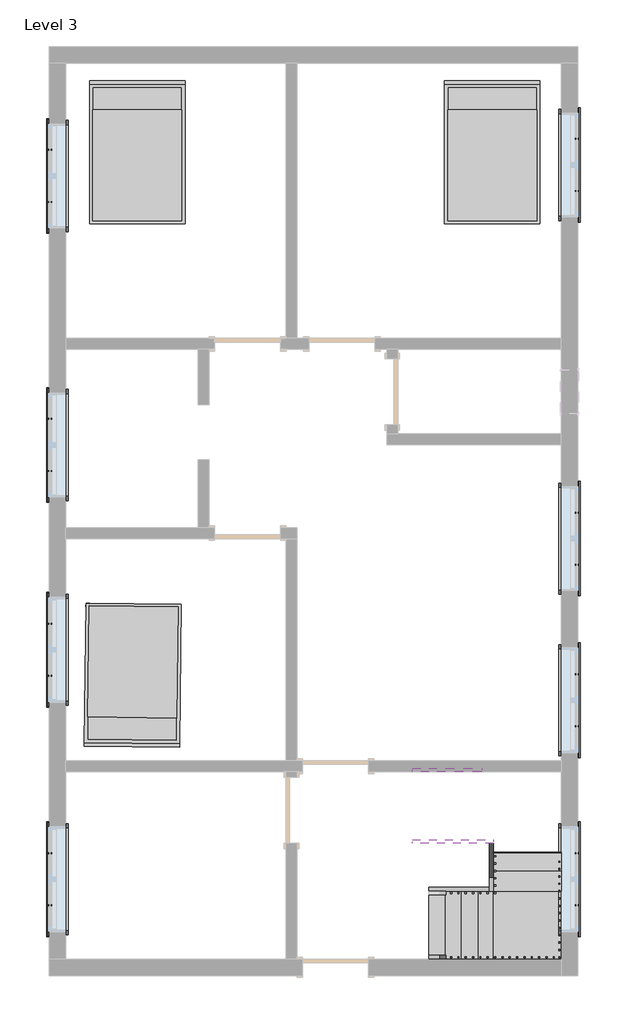
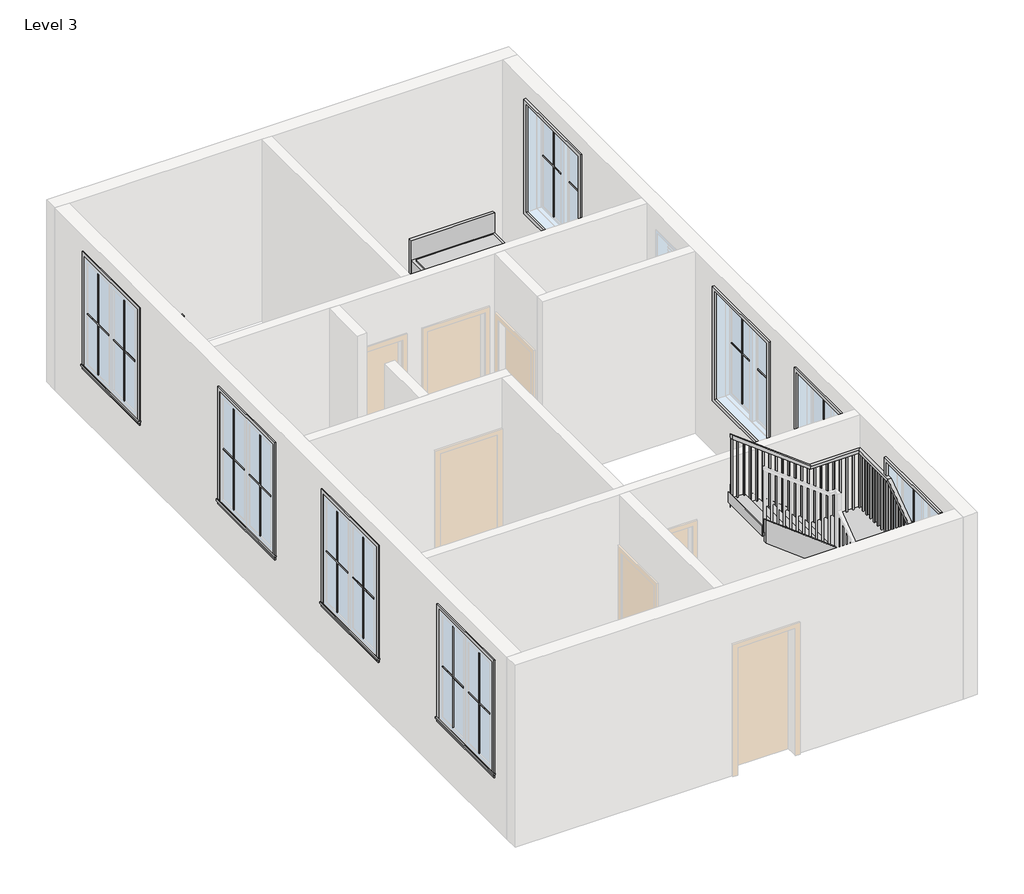
# One storey, part 2 of 2: 32 proxies, 5 members, 3 furniture elements, 1 railing, 1 stair flight.
"""IFC4 building model written with IfcOpenShell, lengths in millimetres."""

from ifc_helpers import new_model, si_unit, frame, origin, place, context, project, spatial, polyline, outline, extrude, faceted_brep, transform, mapped, element, save
from components import muntin_pattern_2x2_muntin_pattern_2x2_bff912c5, muntin_pattern_2x2_muntin_pattern_2x2_c2194282, trim_window_exterior_flat_with_sill_e04b3088, trim_window_interior_flat_picture_frame_2a7685fe, bed_17739_bed_17739_15c61121, stair_flight_84673ee4

model = new_model("IFC4")

# Units and contexts
model_context = context("Model", 3, world=origin())
ifc_project = project(units=[si_unit("LENGTHUNIT", "METRE", prefix="MILLI")], contexts=[model_context])

# Site, building, storey
site = spatial("IfcSite", under=ifc_project)
building = spatial("IfcBuilding", under=site)
storey = spatial("IfcBuildingStorey", under=building, Name="Level 3", Elevation=3200.4)

# Proxies
placement = place(None, origin())
muntin_pattern_2x2_muntin_pattern_2x2_shape = muntin_pattern_2x2_muntin_pattern_2x2_bff912c5(model_context)
element("IfcBuildingElementProxy", 1, Name="Muntin Pattern_2x2 : Muntin Pattern_2x2", ObjectType="Muntin Pattern_2x2 : Muntin Pattern_2x2", at=placement, inside=storey, context=model_context, shape_type="MappedRepresentation", body=[
    mapped(muntin_pattern_2x2_muntin_pattern_2x2_shape, transform((-4903.510885, -5396.5975571, 4184.65), x_axis=(0.0, 1.0, 0.0), y_axis=(-1.0, 0.0, 0.0), z_axis=(0.0, 0.0, 1.0))),
])
element("IfcBuildingElementProxy", 2, Name="Muntin Pattern_2x2 : Muntin Pattern_2x2", ObjectType="Muntin Pattern_2x2 : Muntin Pattern_2x2", at=placement, inside=storey, context=model_context, shape_type="MappedRepresentation", body=[
    mapped(muntin_pattern_2x2_muntin_pattern_2x2_shape, transform((2392.639115, -4675.8725571, 4184.65), x_axis=(0.0, -1.0, 0.0), y_axis=(1.0, 0.0, 0.0), z_axis=(0.0, 0.0, 1.0))),
])
element("IfcBuildingElementProxy", 3, Name="Muntin Pattern_2x2 : Muntin Pattern_2x2", ObjectType="Muntin Pattern_2x2 : Muntin Pattern_2x2", at=placement, inside=storey, context=model_context, shape_type="MappedRepresentation", body=[
    mapped(muntin_pattern_2x2_muntin_pattern_2x2_shape, transform((2392.639115, -2199.3725571, 4184.65), x_axis=(0.0, -1.0, 0.0), y_axis=(1.0, 0.0, 0.0), z_axis=(0.0, 0.0, 1.0))),
])
element("IfcBuildingElementProxy", 4, Name="Muntin Pattern_2x2 : Muntin Pattern_2x2", ObjectType="Muntin Pattern_2x2 : Muntin Pattern_2x2", at=placement, inside=storey, context=model_context, shape_type="MappedRepresentation", body=[
    mapped(muntin_pattern_2x2_muntin_pattern_2x2_shape, transform((2392.639115, 35.8274429, 4184.65), x_axis=(0.0, -1.0, 0.0), y_axis=(1.0, 0.0, 0.0), z_axis=(0.0, 0.0, 1.0))),
])
element("IfcBuildingElementProxy", 5, Name="Muntin Pattern_2x2 : Muntin Pattern_2x2", ObjectType="Muntin Pattern_2x2 : Muntin Pattern_2x2", at=placement, inside=storey, context=model_context, shape_type="MappedRepresentation", body=[
    mapped(muntin_pattern_2x2_muntin_pattern_2x2_shape, transform((-4903.510885, -2221.5975571, 4184.65), x_axis=(0.0, 1.0, 0.0), y_axis=(-1.0, 0.0, 0.0), z_axis=(0.0, 0.0, 1.0))),
])
element("IfcBuildingElementProxy", 6, Name="Muntin Pattern_2x2 : Muntin Pattern_2x2", ObjectType="Muntin Pattern_2x2 : Muntin Pattern_2x2", at=placement, inside=storey, context=model_context, shape_type="MappedRepresentation", body=[
    mapped(muntin_pattern_2x2_muntin_pattern_2x2_shape, transform((-4903.510885, 610.5024429, 4184.65), x_axis=(0.0, 1.0, 0.0), y_axis=(-1.0, 0.0, 0.0), z_axis=(0.0, 0.0, 1.0))),
])
element("IfcBuildingElementProxy", 7, Name="Muntin Pattern_2x2 : Muntin Pattern_2x2", ObjectType="Muntin Pattern_2x2 : Muntin Pattern_2x2", at=placement, inside=storey, context=model_context, shape_type="MappedRepresentation", body=[
    mapped(muntin_pattern_2x2_muntin_pattern_2x2_shape, transform((-4903.510885, 4331.6024429, 4184.65), x_axis=(0.0, 1.0, 0.0), y_axis=(-1.0, 0.0, 0.0), z_axis=(0.0, 0.0, 1.0))),
])
element("IfcBuildingElementProxy", 8, Name="Muntin Pattern_2x2 : Muntin Pattern_2x2", ObjectType="Muntin Pattern_2x2 : Muntin Pattern_2x2", at=placement, inside=storey, context=model_context, shape_type="MappedRepresentation", body=[
    mapped(muntin_pattern_2x2_muntin_pattern_2x2_shape, transform((2392.639115, 5204.7274429, 4184.65), x_axis=(0.0, -1.0, 0.0), y_axis=(1.0, 0.0, 0.0), z_axis=(0.0, 0.0, 1.0))),
])
muntin_pattern_2x2_muntin_pattern_2x2_2_shape = muntin_pattern_2x2_muntin_pattern_2x2_c2194282(model_context)
element("IfcBuildingElementProxy", 9, Name="Muntin Pattern_2x2 : Muntin Pattern_2x2", ObjectType="Muntin Pattern_2x2 : Muntin Pattern_2x2", at=placement, inside=storey, context=model_context, shape_type="MappedRepresentation", body=[
    mapped(muntin_pattern_2x2_muntin_pattern_2x2_2_shape, transform((-4903.510885, -4675.8725571, 4184.65), x_axis=(0.0, -1.0, 0.0), y_axis=(1.0, 0.0, 0.0), z_axis=(0.0, 0.0, 1.0))),
])
element("IfcBuildingElementProxy", 10, Name="Muntin Pattern_2x2 : Muntin Pattern_2x2", ObjectType="Muntin Pattern_2x2 : Muntin Pattern_2x2", at=placement, inside=storey, context=model_context, shape_type="MappedRepresentation", body=[
    mapped(muntin_pattern_2x2_muntin_pattern_2x2_2_shape, transform((2392.639115, -5396.5975571, 4184.65), x_axis=(0.0, 1.0, 0.0), y_axis=(-1.0, 0.0, 0.0), z_axis=(0.0, 0.0, 1.0))),
])
element("IfcBuildingElementProxy", 11, Name="Muntin Pattern_2x2 : Muntin Pattern_2x2", ObjectType="Muntin Pattern_2x2 : Muntin Pattern_2x2", at=placement, inside=storey, context=model_context, shape_type="MappedRepresentation", body=[
    mapped(muntin_pattern_2x2_muntin_pattern_2x2_2_shape, transform((2392.639115, -2920.0975571, 4184.65), x_axis=(0.0, 1.0, 0.0), y_axis=(-1.0, 0.0, 0.0), z_axis=(0.0, 0.0, 1.0))),
])
element("IfcBuildingElementProxy", 12, Name="Muntin Pattern_2x2 : Muntin Pattern_2x2", ObjectType="Muntin Pattern_2x2 : Muntin Pattern_2x2", at=placement, inside=storey, context=model_context, shape_type="MappedRepresentation", body=[
    mapped(muntin_pattern_2x2_muntin_pattern_2x2_2_shape, transform((2392.639115, -684.8975571, 4184.65), x_axis=(0.0, 1.0, 0.0), y_axis=(-1.0, 0.0, 0.0), z_axis=(0.0, 0.0, 1.0))),
])
element("IfcBuildingElementProxy", 13, Name="Muntin Pattern_2x2 : Muntin Pattern_2x2", ObjectType="Muntin Pattern_2x2 : Muntin Pattern_2x2", at=placement, inside=storey, context=model_context, shape_type="MappedRepresentation", body=[
    mapped(muntin_pattern_2x2_muntin_pattern_2x2_2_shape, transform((-4903.510885, -1500.8725571, 4184.65), x_axis=(0.0, -1.0, 0.0), y_axis=(1.0, 0.0, 0.0), z_axis=(0.0, 0.0, 1.0))),
])
element("IfcBuildingElementProxy", 14, Name="Muntin Pattern_2x2 : Muntin Pattern_2x2", ObjectType="Muntin Pattern_2x2 : Muntin Pattern_2x2", at=placement, inside=storey, context=model_context, shape_type="MappedRepresentation", body=[
    mapped(muntin_pattern_2x2_muntin_pattern_2x2_2_shape, transform((-4903.510885, 1331.2274429, 4184.65), x_axis=(0.0, -1.0, 0.0), y_axis=(1.0, 0.0, 0.0), z_axis=(0.0, 0.0, 1.0))),
])
element("IfcBuildingElementProxy", 15, Name="Muntin Pattern_2x2 : Muntin Pattern_2x2", ObjectType="Muntin Pattern_2x2 : Muntin Pattern_2x2", at=placement, inside=storey, context=model_context, shape_type="MappedRepresentation", body=[
    mapped(muntin_pattern_2x2_muntin_pattern_2x2_2_shape, transform((-4903.510885, 5052.3274429, 4184.65), x_axis=(0.0, -1.0, 0.0), y_axis=(1.0, 0.0, 0.0), z_axis=(0.0, 0.0, 1.0))),
])
element("IfcBuildingElementProxy", 16, Name="Muntin Pattern_2x2 : Muntin Pattern_2x2", ObjectType="Muntin Pattern_2x2 : Muntin Pattern_2x2", at=placement, inside=storey, context=model_context, shape_type="MappedRepresentation", body=[
    mapped(muntin_pattern_2x2_muntin_pattern_2x2_2_shape, transform((2392.639115, 4484.0024429, 4184.65), x_axis=(0.0, 1.0, 0.0), y_axis=(-1.0, 0.0, 0.0), z_axis=(0.0, 0.0, 1.0))),
])
trim_window_exterior_flat_with_sill_shape = trim_window_exterior_flat_with_sill_e04b3088(model_context)
element("IfcBuildingElementProxy", 17, Name="Trim-Window-Exterior-Flat : with Sill", ObjectType="Trim-Window-Exterior-Flat : with Sill", at=placement, inside=storey, context=model_context, shape_type="MappedRepresentation", body=[
    mapped(trim_window_exterior_flat_with_sill_shape, transform((-4913.035885, -5036.2350571, 5943.6), x_axis=(0.0, -1.0, 0.0), y_axis=(0.0, 0.0, 1.0), z_axis=(-1.0, 0.0, 0.0))),
])
element("IfcBuildingElementProxy", 18, Name="Trim-Window-Exterior-Flat : with Sill", ObjectType="Trim-Window-Exterior-Flat : with Sill", at=placement, inside=storey, context=model_context, shape_type="MappedRepresentation", body=[
    mapped(trim_window_exterior_flat_with_sill_shape, transform((2402.164115, -5036.2350571, 5943.6), x_axis=(0.0, 1.0, 0.0), y_axis=(0.0, 0.0, 1.0), z_axis=(1.0, 0.0, 0.0))),
])
element("IfcBuildingElementProxy", 19, Name="Trim-Window-Exterior-Flat : with Sill", ObjectType="Trim-Window-Exterior-Flat : with Sill", at=placement, inside=storey, context=model_context, shape_type="MappedRepresentation", body=[
    mapped(trim_window_exterior_flat_with_sill_shape, transform((2402.164115, -2559.7350571, 5943.6), x_axis=(0.0, 1.0, 0.0), y_axis=(0.0, 0.0, 1.0), z_axis=(1.0, 0.0, 0.0))),
])
element("IfcBuildingElementProxy", 20, Name="Trim-Window-Exterior-Flat : with Sill", ObjectType="Trim-Window-Exterior-Flat : with Sill", at=placement, inside=storey, context=model_context, shape_type="MappedRepresentation", body=[
    mapped(trim_window_exterior_flat_with_sill_shape, transform((2402.164115, -324.5350571, 5943.6), x_axis=(0.0, 1.0, 0.0), y_axis=(0.0, 0.0, 1.0), z_axis=(1.0, 0.0, 0.0))),
])
element("IfcBuildingElementProxy", 21, Name="Trim-Window-Exterior-Flat : with Sill", ObjectType="Trim-Window-Exterior-Flat : with Sill", at=placement, inside=storey, context=model_context, shape_type="MappedRepresentation", body=[
    mapped(trim_window_exterior_flat_with_sill_shape, transform((-4913.035885, -1861.2350571, 5943.6), x_axis=(0.0, -1.0, 0.0), y_axis=(0.0, 0.0, 1.0), z_axis=(-1.0, 0.0, 0.0))),
])
element("IfcBuildingElementProxy", 22, Name="Trim-Window-Exterior-Flat : with Sill", ObjectType="Trim-Window-Exterior-Flat : with Sill", at=placement, inside=storey, context=model_context, shape_type="MappedRepresentation", body=[
    mapped(trim_window_exterior_flat_with_sill_shape, transform((-4913.035885, 970.8649429, 5943.6), x_axis=(0.0, -1.0, 0.0), y_axis=(0.0, 0.0, 1.0), z_axis=(-1.0, 0.0, 0.0))),
])
element("IfcBuildingElementProxy", 23, Name="Trim-Window-Exterior-Flat : with Sill", ObjectType="Trim-Window-Exterior-Flat : with Sill", at=placement, inside=storey, context=model_context, shape_type="MappedRepresentation", body=[
    mapped(trim_window_exterior_flat_with_sill_shape, transform((-4913.035885, 4691.9649429, 5943.6), x_axis=(0.0, -1.0, 0.0), y_axis=(0.0, 0.0, 1.0), z_axis=(-1.0, 0.0, 0.0))),
])
element("IfcBuildingElementProxy", 24, Name="Trim-Window-Exterior-Flat : with Sill", ObjectType="Trim-Window-Exterior-Flat : with Sill", at=placement, inside=storey, context=model_context, shape_type="MappedRepresentation", body=[
    mapped(trim_window_exterior_flat_with_sill_shape, transform((2402.164115, 4844.3649429, 5943.6), x_axis=(0.0, 1.0, 0.0), y_axis=(0.0, 0.0, 1.0), z_axis=(1.0, 0.0, 0.0))),
])
trim_window_interior_flat_picture_frame_shape = trim_window_interior_flat_picture_frame_2a7685fe(model_context)
element("IfcBuildingElementProxy", 25, Name="Trim-Window-Interior-Flat : Picture Frame", ObjectType="Trim-Window-Interior-Flat : Picture Frame", at=placement, inside=storey, context=model_context, shape_type="MappedRepresentation", body=[
    mapped(trim_window_interior_flat_picture_frame_shape, transform((-4684.435885, -5036.2350571, 5943.6), x_axis=(0.0, 1.0, 0.0), y_axis=(0.0, 0.0, 1.0), z_axis=(1.0, 0.0, 0.0))),
])
element("IfcBuildingElementProxy", 26, Name="Trim-Window-Interior-Flat : Picture Frame", ObjectType="Trim-Window-Interior-Flat : Picture Frame", at=placement, inside=storey, context=model_context, shape_type="MappedRepresentation", body=[
    mapped(trim_window_interior_flat_picture_frame_shape, transform((2173.564115, -5036.2350571, 5943.6), x_axis=(0.0, -1.0, 0.0), y_axis=(0.0, 0.0, 1.0), z_axis=(-1.0, 0.0, 0.0))),
])
element("IfcBuildingElementProxy", 27, Name="Trim-Window-Interior-Flat : Picture Frame", ObjectType="Trim-Window-Interior-Flat : Picture Frame", at=placement, inside=storey, context=model_context, shape_type="MappedRepresentation", body=[
    mapped(trim_window_interior_flat_picture_frame_shape, transform((2173.564115, -2559.7350571, 5943.6), x_axis=(0.0, -1.0, 0.0), y_axis=(0.0, 0.0, 1.0), z_axis=(-1.0, 0.0, 0.0))),
])
element("IfcBuildingElementProxy", 28, Name="Trim-Window-Interior-Flat : Picture Frame", ObjectType="Trim-Window-Interior-Flat : Picture Frame", at=placement, inside=storey, context=model_context, shape_type="MappedRepresentation", body=[
    mapped(trim_window_interior_flat_picture_frame_shape, transform((2173.564115, -324.5350571, 5943.6), x_axis=(0.0, -1.0, 0.0), y_axis=(0.0, 0.0, 1.0), z_axis=(-1.0, 0.0, 0.0))),
])
element("IfcBuildingElementProxy", 29, Name="Trim-Window-Interior-Flat : Picture Frame", ObjectType="Trim-Window-Interior-Flat : Picture Frame", at=placement, inside=storey, context=model_context, shape_type="MappedRepresentation", body=[
    mapped(trim_window_interior_flat_picture_frame_shape, transform((-4684.435885, -1861.2350571, 5943.6), x_axis=(0.0, 1.0, 0.0), y_axis=(0.0, 0.0, 1.0), z_axis=(1.0, 0.0, 0.0))),
])
element("IfcBuildingElementProxy", 30, Name="Trim-Window-Interior-Flat : Picture Frame", ObjectType="Trim-Window-Interior-Flat : Picture Frame", at=placement, inside=storey, context=model_context, shape_type="MappedRepresentation", body=[
    mapped(trim_window_interior_flat_picture_frame_shape, transform((-4684.435885, 970.8649429, 5943.6), x_axis=(0.0, 1.0, 0.0), y_axis=(0.0, 0.0, 1.0), z_axis=(1.0, 0.0, 0.0))),
])
element("IfcBuildingElementProxy", 31, Name="Trim-Window-Interior-Flat : Picture Frame", ObjectType="Trim-Window-Interior-Flat : Picture Frame", at=placement, inside=storey, context=model_context, shape_type="MappedRepresentation", body=[
    mapped(trim_window_interior_flat_picture_frame_shape, transform((-4684.435885, 4691.9649429, 5943.6), x_axis=(0.0, 1.0, 0.0), y_axis=(0.0, 0.0, 1.0), z_axis=(1.0, 0.0, 0.0))),
])
element("IfcBuildingElementProxy", 32, Name="Trim-Window-Interior-Flat : Picture Frame", ObjectType="Trim-Window-Interior-Flat : Picture Frame", at=placement, inside=storey, context=model_context, shape_type="MappedRepresentation", body=[
    mapped(trim_window_interior_flat_picture_frame_shape, transform((2173.564115, 4844.3649429, 5943.6), x_axis=(0.0, -1.0, 0.0), y_axis=(0.0, 0.0, 1.0), z_axis=(-1.0, 0.0, 0.0))),
])

# Furniture
bed_17739_bed_17739_shape = bed_17739_bed_17739_15c61121(model_context)
element("IfcFurniture", 33, ObjectType="Bed_17739 : Bed_17739", at=placement, inside=storey, context=model_context, shape_type="MappedRepresentation", body=[
    mapped(bed_17739_bed_17739_shape, transform((-3693.835885, 4996.7649429, 3200.4), x_axis=(1.0, 0.0, 0.0), y_axis=(0.0, 1.0, 0.0), z_axis=(0.0, 0.0, 1.0))),
])
element("IfcFurniture", 34, ObjectType="Bed_17739 : Bed_17739", at=placement, inside=storey, context=model_context, shape_type="MappedRepresentation", body=[
    mapped(bed_17739_bed_17739_shape, transform((1221.064115, 4996.7649429, 3200.4), x_axis=(1.0, 0.0, 0.0), y_axis=(0.0, 1.0, 0.0), z_axis=(0.0, 0.0, 1.0))),
])
element("IfcFurniture", 35, ObjectType="Bed_17739 : Bed_17739", at=placement, inside=storey, context=model_context, shape_type="MappedRepresentation", body=[
    mapped(bed_17739_bed_17739_shape, transform((-3756.0321663, -2189.364606, 3200.4), x_axis=(-0.9999334593473937, 0.011535895177843815, 0.0), y_axis=(-0.011535895177843815, -0.9999334593473937, 0.0), z_axis=(0.0, 0.0, 1.0))),
])

# Members
element("IfcMember", 36, ObjectType="Stringer - 2\" Width", at=placement, inside=storey, context=model_context, shape_type="SweptSolid", body=[
    extrude(outline(polyline([(3423.0959685, 344.764115), (3200.4, 344.764115), (3200.4, 555.1685253), (3683.3196844, 1182.964115), (4067.8651993, 1182.964115), (3423.0959685, 344.764115)])), frame((0.0, -5201.3350571, 0.0), z_axis=(0.0, 1.0, 0.0), x_axis=(0.0, 0.0, 1.0)), (0.0, 0.0, 1.0), 50.8),
])
element("IfcMember", 37, ObjectType="Stringer - 2\" Width", at=placement, inside=storey, context=model_context, shape_type="SweptSolid", body=[
    extrude(outline(polyline([(-5201.3350571, 3895.552716), (-5201.3350571, 4270.1225362), (-4540.9350571, 4741.8368219), (-4540.9350571, 4367.2670017), (-5201.3350571, 3895.552716)])), frame((1182.964115, 0.0, 0.0), z_axis=(1.0, 0.0, 0.0), x_axis=(0.0, 1.0, 0.0)), (0.0, 0.0, 1.0), 50.8),
])
element("IfcMember", 38, ObjectType="Stringer - 2\" Width", at=placement, inside=storey, context=model_context, shape_type="SweptSolid", body=[
    extrude(outline(polyline([(4569.5786616, 1233.764115), (4952.7668, 1233.764115), (5804.2715619, 116.164115), (5421.0834236, 116.164115), (4569.5786616, 1233.764115)])), frame((0.0, -4540.9350571, 0.0), z_axis=(0.0, 1.0, 0.0), x_axis=(0.0, 0.0, 1.0)), (0.0, 0.0, 1.0), 50.8),
])
element("IfcMember", 39, ObjectType="Stringer - 2\" Width", at=placement, inside=storey, context=model_context, shape_type="SweptSolid", body=[
    extrude(outline(polyline([(3423.0959685, 344.764115), (3200.4, 344.764115), (3200.4, 555.1685253), (3598.8368219, 1073.1363938), (3598.8368219, 573.2272245), (3423.0959685, 344.764115)])), frame((0.0, -6191.9350571, 0.0), z_axis=(0.0, 1.0, 0.0), x_axis=(0.0, 0.0, 1.0)), (0.0, 0.0, 1.0), 50.8),
])
element("IfcMember", 40, ObjectType="Stringer - 2\" Width", at=placement, inside=storey, context=model_context, shape_type="SweptSolid", body=[
    extrude(outline(polyline([(5074.8384303, 1073.5451003), (5804.2715619, 116.164115), (5421.0834236, 116.164115), (5074.8384303, 570.6106687), (5074.8384303, 1073.5451003)])), frame((0.0, -3550.3350571, 0.0), z_axis=(0.0, 1.0, 0.0), x_axis=(0.0, 0.0, 1.0)), (0.0, 0.0, 1.0), 50.8),
])

# Railing
element("IfcRailing", 41, ObjectType="Handrail - Rectangular", at=placement, inside=storey, context=model_context, shape_type="SolidModel", body=[
    faceted_brep([(344.764115, -6090.3350571, 4284.1333333), (344.764115, -6090.3350571, 4220.2686436), (344.764115, -6141.1350571, 4220.2686436), (344.764115, -6141.1350571, 4284.1333333), (1373.464115, -6090.3350571, 5067.9047619), (1390.6115203, -6090.3350571, 5017.1047619), (1390.6115203, -6141.1350571, 5017.1047619), (1373.464115, -6141.1350571, 5067.9047619), (2122.764115, -6090.3350571, 5067.9047619), (2122.764115, -6090.3350571, 5017.1047619), (2173.564115, -6141.1350571, 5017.1047619), (2173.564115, -6141.1350571, 5067.9047619), (2122.764115, -5289.3883904, 5067.9047619), (2122.764115, -5273.1087657, 5017.1047619), (2173.564115, -5273.1087657, 5017.1047619), (2173.564115, -5289.3883904, 5067.9047619), (2122.764115, -4399.3108146, 5703.6744589), (2122.764115, -4383.0311899, 5652.8744589), (2173.564115, -4383.0311899, 5652.8744589), (2173.564115, -4399.3108146, 5703.6744589), (2122.764115, -3601.1350571, 5703.6744589), (2122.764115, -3601.1350571, 5652.8744589), (2173.564115, -3550.3350571, 5652.8744589), (2173.564115, -3550.3350571, 5703.6744589), (1371.6498293, -3601.1350571, 5703.6744589), (1354.5800477, -3601.1350571, 5652.8744589), (1354.5800477, -3550.3350571, 5652.8744589), (1371.6498293, -3550.3350571, 5703.6744589), (116.164115, -3601.1350571, 6654.8), (116.164115, -3550.3350571, 6654.8), (116.164115, -3550.3350571, 6591.0683472), (116.164115, -3601.1350571, 6591.0683472)], [[[0, 1, 2, 3]], [[1, 0, 4, 5]], [[2, 1, 5, 6]], [[3, 2, 6, 7]], [[0, 3, 7, 4]], [[5, 4, 8, 9]], [[6, 5, 9, 10]], [[7, 6, 10, 11]], [[4, 7, 11, 8]], [[9, 8, 12, 13]], [[10, 9, 13, 14]], [[11, 10, 14, 15]], [[8, 11, 15, 12]], [[13, 12, 16, 17]], [[14, 13, 17, 18]], [[15, 14, 18, 19]], [[12, 15, 19, 16]], [[17, 16, 20, 21]], [[18, 17, 21, 22]], [[19, 18, 22, 23]], [[16, 19, 23, 20]], [[21, 20, 24, 25]], [[22, 21, 25, 26]], [[23, 22, 26, 27]], [[20, 23, 27, 24]], [[28, 29, 30, 31]], [[25, 24, 28, 31]], [[26, 25, 31, 30]], [[27, 26, 30, 29]], [[24, 27, 29, 28]]]),
    extrude(outline(polyline([(6506.8827412, 227.289115), (6521.3145594, 208.239115), (5571.0666667, 208.239115), (5571.0666667, 227.289115), (6506.8827412, 227.289115)])), frame((0.0, -3585.2600571, 0.0), z_axis=(0.0, 1.0, 0.0), x_axis=(0.0, 0.0, 1.0)), (0.0, 0.0, 1.0), 19.05),
    extrude(outline(polyline([(6429.9130442, 328.889115), (6444.3448624, 309.839115), (5571.0666667, 309.839115), (5571.0666667, 328.889115), (6429.9130442, 328.889115)])), frame((0.0, -3585.2600571, 0.0), z_axis=(0.0, 1.0, 0.0), x_axis=(0.0, 0.0, 1.0)), (0.0, 0.0, 1.0), 19.05),
    extrude(outline(polyline([(6352.9433472, 430.489115), (6367.3751654, 411.439115), (5401.7333333, 411.439115), (5401.7333333, 430.489115), (6352.9433472, 430.489115)])), frame((0.0, -3585.2600571, 0.0), z_axis=(0.0, 1.0, 0.0), x_axis=(0.0, 0.0, 1.0)), (0.0, 0.0, 1.0), 19.05),
    extrude(outline(polyline([(6275.9736503, 532.089115), (6290.4054685, 513.039115), (5401.7333333, 513.039115), (5401.7333333, 532.089115), (6275.9736503, 532.089115)])), frame((0.0, -3585.2600571, 0.0), z_axis=(0.0, 1.0, 0.0), x_axis=(0.0, 0.0, 1.0)), (0.0, 0.0, 1.0), 19.05),
    extrude(outline(polyline([(6199.0039533, 633.689115), (6213.4357715, 614.639115), (5232.4, 614.639115), (5232.4, 633.689115), (6199.0039533, 633.689115)])), frame((0.0, -3585.2600571, 0.0), z_axis=(0.0, 1.0, 0.0), x_axis=(0.0, 0.0, 1.0)), (0.0, 0.0, 1.0), 19.05),
    extrude(outline(polyline([(6122.0342563, 735.289115), (6136.4660745, 716.239115), (5232.4, 716.239115), (5232.4, 735.289115), (6122.0342563, 735.289115)])), frame((0.0, -3585.2600571, 0.0), z_axis=(0.0, 1.0, 0.0), x_axis=(0.0, 0.0, 1.0)), (0.0, 0.0, 1.0), 19.05),
    extrude(outline(polyline([(6045.0645594, 836.889115), (6059.4963775, 817.839115), (5063.0666667, 817.839115), (5063.0666667, 836.889115), (6045.0645594, 836.889115)])), frame((0.0, -3585.2600571, 0.0), z_axis=(0.0, 1.0, 0.0), x_axis=(0.0, 0.0, 1.0)), (0.0, 0.0, 1.0), 19.05),
    extrude(outline(polyline([(5968.0948624, 938.489115), (5982.5266806, 919.439115), (5063.0666667, 919.439115), (5063.0666667, 938.489115), (5968.0948624, 938.489115)])), frame((0.0, -3585.2600571, 0.0), z_axis=(0.0, 1.0, 0.0), x_axis=(0.0, 0.0, 1.0)), (0.0, 0.0, 1.0), 19.05),
    extrude(outline(polyline([(5891.1251654, 1040.089115), (5905.5569836, 1021.039115), (5063.0666667, 1021.039115), (5063.0666667, 1040.089115), (5891.1251654, 1040.089115)])), frame((0.0, -3585.2600571, 0.0), z_axis=(0.0, 1.0, 0.0), x_axis=(0.0, 0.0, 1.0)), (0.0, 0.0, 1.0), 19.05),
    extrude(outline(polyline([(5814.1554685, 1141.689115), (5828.5872866, 1122.639115), (4893.7333333, 1122.639115), (4893.7333333, 1141.689115), (5814.1554685, 1141.689115)])), frame((0.0, -3585.2600571, 0.0), z_axis=(0.0, 1.0, 0.0), x_axis=(0.0, 0.0, 1.0)), (0.0, 0.0, 1.0), 19.05),
    extrude(outline(polyline([(5737.1857715, 1243.289115), (5751.6175897, 1224.239115), (4893.7333333, 1224.239115), (4893.7333333, 1243.289115), (5737.1857715, 1243.289115)])), frame((0.0, -3585.2600571, 0.0), z_axis=(0.0, 1.0, 0.0), x_axis=(0.0, 0.0, 1.0)), (0.0, 0.0, 1.0), 19.05),
    extrude(outline(polyline([(5660.2160745, 1344.889115), (5674.6478927, 1325.839115), (4724.4, 1325.839115), (4724.4, 1344.889115), (5660.2160745, 1344.889115)])), frame((0.0, -3585.2600571, 0.0), z_axis=(0.0, 1.0, 0.0), x_axis=(0.0, 0.0, 1.0)), (0.0, 0.0, 1.0), 19.05),
    extrude(outline(polyline([(1446.489115, -3566.2100571), (1446.489115, -3585.2600571), (1427.439115, -3585.2600571), (1427.439115, -3566.2100571), (1446.489115, -3566.2100571)])), frame((0.0, 0.0, 4724.4), z_axis=(0.0, 0.0, 1.0), x_axis=(1.0, 0.0, 0.0)), (0.0, 0.0, 1.0), 928.4744589),
    extrude(outline(polyline([(1548.089115, -3566.2100571), (1548.089115, -3585.2600571), (1529.039115, -3585.2600571), (1529.039115, -3566.2100571), (1548.089115, -3566.2100571)])), frame((0.0, 0.0, 4724.4), z_axis=(0.0, 0.0, 1.0), x_axis=(1.0, 0.0, 0.0)), (0.0, 0.0, 1.0), 928.4744589),
    extrude(outline(polyline([(1649.689115, -3566.2100571), (1649.689115, -3585.2600571), (1630.639115, -3585.2600571), (1630.639115, -3566.2100571), (1649.689115, -3566.2100571)])), frame((0.0, 0.0, 4724.4), z_axis=(0.0, 0.0, 1.0), x_axis=(1.0, 0.0, 0.0)), (0.0, 0.0, 1.0), 928.4744589),
    extrude(outline(polyline([(1751.289115, -3566.2100571), (1751.289115, -3585.2600571), (1732.239115, -3585.2600571), (1732.239115, -3566.2100571), (1751.289115, -3566.2100571)])), frame((0.0, 0.0, 4724.4), z_axis=(0.0, 0.0, 1.0), x_axis=(1.0, 0.0, 0.0)), (0.0, 0.0, 1.0), 928.4744589),
    extrude(outline(polyline([(1852.889115, -3566.2100571), (1852.889115, -3585.2600571), (1833.839115, -3585.2600571), (1833.839115, -3566.2100571), (1852.889115, -3566.2100571)])), frame((0.0, 0.0, 4724.4), z_axis=(0.0, 0.0, 1.0), x_axis=(1.0, 0.0, 0.0)), (0.0, 0.0, 1.0), 928.4744589),
    extrude(outline(polyline([(1954.489115, -3566.2100571), (1954.489115, -3585.2600571), (1935.439115, -3585.2600571), (1935.439115, -3566.2100571), (1954.489115, -3566.2100571)])), frame((0.0, 0.0, 4724.4), z_axis=(0.0, 0.0, 1.0), x_axis=(1.0, 0.0, 0.0)), (0.0, 0.0, 1.0), 928.4744589),
    extrude(outline(polyline([(2056.089115, -3566.2100571), (2056.089115, -3585.2600571), (2037.039115, -3585.2600571), (2037.039115, -3566.2100571), (2056.089115, -3566.2100571)])), frame((0.0, 0.0, 4724.4), z_axis=(0.0, 0.0, 1.0), x_axis=(1.0, 0.0, 0.0)), (0.0, 0.0, 1.0), 928.4744589),
    extrude(outline(polyline([(2157.689115, -3686.8600571), (2138.639115, -3686.8600571), (2138.639115, -3667.8100571), (2157.689115, -3667.8100571), (2157.689115, -3686.8600571)])), frame((0.0, 0.0, 4724.4), z_axis=(0.0, 0.0, 1.0), x_axis=(1.0, 0.0, 0.0)), (0.0, 0.0, 1.0), 928.4744589),
    extrude(outline(polyline([(2157.689115, -3788.4600571), (2138.639115, -3788.4600571), (2138.639115, -3769.4100571), (2157.689115, -3769.4100571), (2157.689115, -3788.4600571)])), frame((0.0, 0.0, 4724.4), z_axis=(0.0, 0.0, 1.0), x_axis=(1.0, 0.0, 0.0)), (0.0, 0.0, 1.0), 928.4744589),
    extrude(outline(polyline([(2157.689115, -3890.0600571), (2138.639115, -3890.0600571), (2138.639115, -3871.0100571), (2157.689115, -3871.0100571), (2157.689115, -3890.0600571)])), frame((0.0, 0.0, 4724.4), z_axis=(0.0, 0.0, 1.0), x_axis=(1.0, 0.0, 0.0)), (0.0, 0.0, 1.0), 928.4744589),
    extrude(outline(polyline([(2157.689115, -3991.6600571), (2138.639115, -3991.6600571), (2138.639115, -3972.6100571), (2157.689115, -3972.6100571), (2157.689115, -3991.6600571)])), frame((0.0, 0.0, 4724.4), z_axis=(0.0, 0.0, 1.0), x_axis=(1.0, 0.0, 0.0)), (0.0, 0.0, 1.0), 928.4744589),
    extrude(outline(polyline([(2157.689115, -4093.2600571), (2138.639115, -4093.2600571), (2138.639115, -4074.2100571), (2157.689115, -4074.2100571), (2157.689115, -4093.2600571)])), frame((0.0, 0.0, 4724.4), z_axis=(0.0, 0.0, 1.0), x_axis=(1.0, 0.0, 0.0)), (0.0, 0.0, 1.0), 928.4744589),
    extrude(outline(polyline([(2157.689115, -4194.8600571), (2138.639115, -4194.8600571), (2138.639115, -4175.8100571), (2157.689115, -4175.8100571), (2157.689115, -4194.8600571)])), frame((0.0, 0.0, 4724.4), z_axis=(0.0, 0.0, 1.0), x_axis=(1.0, 0.0, 0.0)), (0.0, 0.0, 1.0), 928.4744589),
    extrude(outline(polyline([(2157.689115, -4296.4600571), (2138.639115, -4296.4600571), (2138.639115, -4277.4100571), (2157.689115, -4277.4100571), (2157.689115, -4296.4600571)])), frame((0.0, 0.0, 4724.4), z_axis=(0.0, 0.0, 1.0), x_axis=(1.0, 0.0, 0.0)), (0.0, 0.0, 1.0), 928.4744589),
    extrude(outline(polyline([(2157.689115, -4398.0600571), (2138.639115, -4398.0600571), (2138.639115, -4379.0100571), (2157.689115, -4379.0100571), (2157.689115, -4398.0600571)])), frame((0.0, 0.0, 4724.4), z_axis=(0.0, 0.0, 1.0), x_axis=(1.0, 0.0, 0.0)), (0.0, 0.0, 1.0), 928.4744589),
    extrude(outline(polyline([(-4499.6600571, 5569.5681252), (-4480.6100571, 5583.1752681), (-4480.6100571, 4724.4), (-4499.6600571, 4724.4), (-4499.6600571, 5569.5681252)])), frame((2138.639115, 0.0, 0.0), z_axis=(1.0, 0.0, 0.0), x_axis=(0.0, 1.0, 0.0)), (0.0, 0.0, 1.0), 19.05),
    extrude(outline(polyline([(-4601.2600571, 5496.9966966), (-4582.2100571, 5510.6038395), (-4582.2100571, 4555.0666667), (-4601.2600571, 4555.0666667), (-4601.2600571, 5496.9966966)])), frame((2138.639115, 0.0, 0.0), z_axis=(1.0, 0.0, 0.0), x_axis=(0.0, 1.0, 0.0)), (0.0, 0.0, 1.0), 19.05),
    extrude(outline(polyline([(-4702.8600571, 5424.4252681), (-4683.8100571, 5438.0324109), (-4683.8100571, 4555.0666667), (-4702.8600571, 4555.0666667), (-4702.8600571, 5424.4252681)])), frame((2138.639115, 0.0, 0.0), z_axis=(1.0, 0.0, 0.0), x_axis=(0.0, 1.0, 0.0)), (0.0, 0.0, 1.0), 19.05),
    extrude(outline(polyline([(-4804.4600571, 5351.8538395), (-4785.4100571, 5365.4609823), (-4785.4100571, 4385.7333333), (-4804.4600571, 4385.7333333), (-4804.4600571, 5351.8538395)])), frame((2138.639115, 0.0, 0.0), z_axis=(1.0, 0.0, 0.0), x_axis=(0.0, 1.0, 0.0)), (0.0, 0.0, 1.0), 19.05),
    extrude(outline(polyline([(-4906.0600571, 5279.2824109), (-4887.0100571, 5292.8895538), (-4887.0100571, 4385.7333333), (-4906.0600571, 4385.7333333), (-4906.0600571, 5279.2824109)])), frame((2138.639115, 0.0, 0.0), z_axis=(1.0, 0.0, 0.0), x_axis=(0.0, 1.0, 0.0)), (0.0, 0.0, 1.0), 19.05),
    extrude(outline(polyline([(-5007.6600571, 5206.7109823), (-4988.6100571, 5220.3181252), (-4988.6100571, 4216.4), (-5007.6600571, 4216.4), (-5007.6600571, 5206.7109823)])), frame((2138.639115, 0.0, 0.0), z_axis=(1.0, 0.0, 0.0), x_axis=(0.0, 1.0, 0.0)), (0.0, 0.0, 1.0), 19.05),
    extrude(outline(polyline([(-5109.2600571, 5134.1395538), (-5090.2100571, 5147.7466966), (-5090.2100571, 4216.4), (-5109.2600571, 4216.4), (-5109.2600571, 5134.1395538)])), frame((2138.639115, 0.0, 0.0), z_axis=(1.0, 0.0, 0.0), x_axis=(0.0, 1.0, 0.0)), (0.0, 0.0, 1.0), 19.05),
    extrude(outline(polyline([(-5210.8600571, 5061.5681252), (-5191.8100571, 5075.1752681), (-5191.8100571, 4216.4), (-5210.8600571, 4216.4), (-5210.8600571, 5061.5681252)])), frame((2138.639115, 0.0, 0.0), z_axis=(1.0, 0.0, 0.0), x_axis=(0.0, 1.0, 0.0)), (0.0, 0.0, 1.0), 19.05),
    extrude(outline(polyline([(2157.689115, -5312.4600571), (2138.639115, -5312.4600571), (2138.639115, -5293.4100571), (2157.689115, -5293.4100571), (2157.689115, -5312.4600571)])), frame((0.0, 0.0, 4047.0666667), z_axis=(0.0, 0.0, 1.0), x_axis=(1.0, 0.0, 0.0)), (0.0, 0.0, 1.0), 970.0380952),
    extrude(outline(polyline([(2157.689115, -5414.0600571), (2138.639115, -5414.0600571), (2138.639115, -5395.0100571), (2157.689115, -5395.0100571), (2157.689115, -5414.0600571)])), frame((0.0, 0.0, 4047.0666667), z_axis=(0.0, 0.0, 1.0), x_axis=(1.0, 0.0, 0.0)), (0.0, 0.0, 1.0), 970.0380952),
    extrude(outline(polyline([(2157.689115, -5515.6600571), (2138.639115, -5515.6600571), (2138.639115, -5496.6100571), (2157.689115, -5496.6100571), (2157.689115, -5515.6600571)])), frame((0.0, 0.0, 4047.0666667), z_axis=(0.0, 0.0, 1.0), x_axis=(1.0, 0.0, 0.0)), (0.0, 0.0, 1.0), 970.0380952),
    extrude(outline(polyline([(2157.689115, -5617.2600571), (2138.639115, -5617.2600571), (2138.639115, -5598.2100571), (2157.689115, -5598.2100571), (2157.689115, -5617.2600571)])), frame((0.0, 0.0, 4047.0666667), z_axis=(0.0, 0.0, 1.0), x_axis=(1.0, 0.0, 0.0)), (0.0, 0.0, 1.0), 970.0380952),
    extrude(outline(polyline([(2157.689115, -5718.8600571), (2138.639115, -5718.8600571), (2138.639115, -5699.8100571), (2157.689115, -5699.8100571), (2157.689115, -5718.8600571)])), frame((0.0, 0.0, 4047.0666667), z_axis=(0.0, 0.0, 1.0), x_axis=(1.0, 0.0, 0.0)), (0.0, 0.0, 1.0), 970.0380952),
    extrude(outline(polyline([(2157.689115, -5820.4600571), (2138.639115, -5820.4600571), (2138.639115, -5801.4100571), (2157.689115, -5801.4100571), (2157.689115, -5820.4600571)])), frame((0.0, 0.0, 4047.0666667), z_axis=(0.0, 0.0, 1.0), x_axis=(1.0, 0.0, 0.0)), (0.0, 0.0, 1.0), 970.0380952),
    extrude(outline(polyline([(2157.689115, -5922.0600571), (2138.639115, -5922.0600571), (2138.639115, -5903.0100571), (2157.689115, -5903.0100571), (2157.689115, -5922.0600571)])), frame((0.0, 0.0, 4047.0666667), z_axis=(0.0, 0.0, 1.0), x_axis=(1.0, 0.0, 0.0)), (0.0, 0.0, 1.0), 970.0380952),
    extrude(outline(polyline([(2157.689115, -6023.6600571), (2138.639115, -6023.6600571), (2138.639115, -6004.6100571), (2157.689115, -6004.6100571), (2157.689115, -6023.6600571)])), frame((0.0, 0.0, 4047.0666667), z_axis=(0.0, 0.0, 1.0), x_axis=(1.0, 0.0, 0.0)), (0.0, 0.0, 1.0), 970.0380952),
    extrude(outline(polyline([(2062.439115, -6125.2600571), (2062.439115, -6106.2100571), (2081.489115, -6106.2100571), (2081.489115, -6125.2600571), (2062.439115, -6125.2600571)])), frame((0.0, 0.0, 4047.0666667), z_axis=(0.0, 0.0, 1.0), x_axis=(1.0, 0.0, 0.0)), (0.0, 0.0, 1.0), 970.0380952),
    extrude(outline(polyline([(1960.839115, -6125.2600571), (1960.839115, -6106.2100571), (1979.889115, -6106.2100571), (1979.889115, -6125.2600571), (1960.839115, -6125.2600571)])), frame((0.0, 0.0, 4047.0666667), z_axis=(0.0, 0.0, 1.0), x_axis=(1.0, 0.0, 0.0)), (0.0, 0.0, 1.0), 970.0380952),
    extrude(outline(polyline([(1859.239115, -6125.2600571), (1859.239115, -6106.2100571), (1878.289115, -6106.2100571), (1878.289115, -6125.2600571), (1859.239115, -6125.2600571)])), frame((0.0, 0.0, 4047.0666667), z_axis=(0.0, 0.0, 1.0), x_axis=(1.0, 0.0, 0.0)), (0.0, 0.0, 1.0), 970.0380952),
    extrude(outline(polyline([(1757.639115, -6125.2600571), (1757.639115, -6106.2100571), (1776.689115, -6106.2100571), (1776.689115, -6125.2600571), (1757.639115, -6125.2600571)])), frame((0.0, 0.0, 4047.0666667), z_axis=(0.0, 0.0, 1.0), x_axis=(1.0, 0.0, 0.0)), (0.0, 0.0, 1.0), 970.0380952),
    extrude(outline(polyline([(1656.039115, -6125.2600571), (1656.039115, -6106.2100571), (1675.089115, -6106.2100571), (1675.089115, -6125.2600571), (1656.039115, -6125.2600571)])), frame((0.0, 0.0, 4047.0666667), z_axis=(0.0, 0.0, 1.0), x_axis=(1.0, 0.0, 0.0)), (0.0, 0.0, 1.0), 970.0380952),
    extrude(outline(polyline([(1554.439115, -6125.2600571), (1554.439115, -6106.2100571), (1573.489115, -6106.2100571), (1573.489115, -6125.2600571), (1554.439115, -6125.2600571)])), frame((0.0, 0.0, 4047.0666667), z_axis=(0.0, 0.0, 1.0), x_axis=(1.0, 0.0, 0.0)), (0.0, 0.0, 1.0), 970.0380952),
    extrude(outline(polyline([(1452.839115, -6125.2600571), (1452.839115, -6106.2100571), (1471.889115, -6106.2100571), (1471.889115, -6125.2600571), (1452.839115, -6125.2600571)])), frame((0.0, 0.0, 4047.0666667), z_axis=(0.0, 0.0, 1.0), x_axis=(1.0, 0.0, 0.0)), (0.0, 0.0, 1.0), 970.0380952),
    extrude(outline(polyline([(5001.6210246, 1370.289115), (4987.1067388, 1351.239115), (4047.0666667, 1351.239115), (4047.0666667, 1370.289115), (5001.6210246, 1370.289115)])), frame((0.0, -6125.2600571, 0.0), z_axis=(0.0, 1.0, 0.0), x_axis=(0.0, 0.0, 1.0)), (0.0, 0.0, 1.0), 19.05),
    extrude(outline(polyline([(4924.2115007, 1268.689115), (4909.697215, 1249.639115), (4047.0666667, 1249.639115), (4047.0666667, 1268.689115), (4924.2115007, 1268.689115)])), frame((0.0, -6125.2600571, 0.0), z_axis=(0.0, 1.0, 0.0), x_axis=(0.0, 0.0, 1.0)), (0.0, 0.0, 1.0), 19.05),
    extrude(outline(polyline([(4846.8019769, 1167.089115), (4832.2876912, 1148.039115), (3877.7333333, 1148.039115), (3877.7333333, 1167.089115), (4846.8019769, 1167.089115)])), frame((0.0, -6125.2600571, 0.0), z_axis=(0.0, 1.0, 0.0), x_axis=(0.0, 0.0, 1.0)), (0.0, 0.0, 1.0), 19.05),
    extrude(outline(polyline([(4769.3924531, 1065.489115), (4754.8781674, 1046.439115), (3877.7333333, 1046.439115), (3877.7333333, 1065.489115), (4769.3924531, 1065.489115)])), frame((0.0, -6125.2600571, 0.0), z_axis=(0.0, 1.0, 0.0), x_axis=(0.0, 0.0, 1.0)), (0.0, 0.0, 1.0), 19.05),
    extrude(outline(polyline([(4691.9829293, 963.889115), (4677.4686436, 944.839115), (3708.4, 944.839115), (3708.4, 963.889115), (4691.9829293, 963.889115)])), frame((0.0, -6125.2600571, 0.0), z_axis=(0.0, 1.0, 0.0), x_axis=(0.0, 0.0, 1.0)), (0.0, 0.0, 1.0), 19.05),
    extrude(outline(polyline([(4614.5734055, 862.289115), (4600.0591198, 843.239115), (3708.4, 843.239115), (3708.4, 862.289115), (4614.5734055, 862.289115)])), frame((0.0, -6125.2600571, 0.0), z_axis=(0.0, 1.0, 0.0), x_axis=(0.0, 0.0, 1.0)), (0.0, 0.0, 1.0), 19.05),
    extrude(outline(polyline([(4537.1638817, 760.689115), (4522.649596, 741.639115), (3539.0666667, 741.639115), (3539.0666667, 760.689115), (4537.1638817, 760.689115)])), frame((0.0, -6125.2600571, 0.0), z_axis=(0.0, 1.0, 0.0), x_axis=(0.0, 0.0, 1.0)), (0.0, 0.0, 1.0), 19.05),
    extrude(outline(polyline([(4459.7543579, 659.089115), (4445.2400722, 640.039115), (3539.0666667, 640.039115), (3539.0666667, 659.089115), (4459.7543579, 659.089115)])), frame((0.0, -6125.2600571, 0.0), z_axis=(0.0, 1.0, 0.0), x_axis=(0.0, 0.0, 1.0)), (0.0, 0.0, 1.0), 19.05),
    extrude(outline(polyline([(4382.3448341, 557.489115), (4367.8305484, 538.439115), (3369.7333333, 538.439115), (3369.7333333, 557.489115), (4382.3448341, 557.489115)])), frame((0.0, -6125.2600571, 0.0), z_axis=(0.0, 1.0, 0.0), x_axis=(0.0, 0.0, 1.0)), (0.0, 0.0, 1.0), 19.05),
    extrude(outline(polyline([(4304.9353103, 455.889115), (4290.4210246, 436.839115), (3369.7333333, 436.839115), (3369.7333333, 455.889115), (4304.9353103, 455.889115)])), frame((0.0, -6125.2600571, 0.0), z_axis=(0.0, 1.0, 0.0), x_axis=(0.0, 0.0, 1.0)), (0.0, 0.0, 1.0), 19.05),
    extrude(outline(polyline([(2157.689115, -3585.2600571), (2138.639115, -3585.2600571), (2138.639115, -3566.2100571), (2157.689115, -3566.2100571), (2157.689115, -3585.2600571)])), frame((0.0, 0.0, 4724.4), z_axis=(0.0, 0.0, 1.0), x_axis=(1.0, 0.0, 0.0)), (0.0, 0.0, 1.0), 928.4744589),
    extrude(outline(polyline([(2138.639115, -6125.2600571), (2138.639115, -6106.2100571), (2157.689115, -6106.2100571), (2157.689115, -6125.2600571), (2138.639115, -6125.2600571)])), frame((0.0, 0.0, 4047.0666667), z_axis=(0.0, 0.0, 1.0), x_axis=(1.0, 0.0, 0.0)), (0.0, 0.0, 1.0), 970.0380952),
    extrude(outline(polyline([(6576.6365291, 135.214115), (6591.0683472, 116.164115), (5571.0666667, 116.164115), (5571.0666667, 135.214115), (6576.6365291, 135.214115)])), frame((0.0, -3585.2600571, 0.0), z_axis=(0.0, 1.0, 0.0), x_axis=(0.0, 0.0, 1.0)), (0.0, 0.0, 1.0), 19.05),
    extrude(outline(polyline([(4234.7829293, 363.814115), (4220.2686436, 344.764115), (3369.7333333, 344.764115), (3369.7333333, 363.814115), (4234.7829293, 363.814115)])), frame((0.0, -6125.2600571, 0.0), z_axis=(0.0, 1.0, 0.0), x_axis=(0.0, 0.0, 1.0)), (0.0, 0.0, 1.0), 19.05),
])

# Stair flight
stair_flight_shape = stair_flight_84673ee4(model_context)
element("IfcStairFlight", 42, ObjectType="2\" Tread 1\" Nosing 1/4\" Riser", at=placement, inside=storey, context=model_context, shape_type="MappedRepresentation", body=[
    mapped(stair_flight_shape, transform((0.0, 0.0, 0.0), x_axis=(1.0, 0.0, 0.0), y_axis=(0.0, 1.0, 0.0), z_axis=(0.0, 0.0, 1.0))),
])

save(model, "model.ifc")

# Revit data of these elements
# Type "Muntin Pattern_2x2 : Muntin Pattern_2x2"
#   Width [instance default] = 4' - 0"
#   Thickness = 0' - 0 1/2"
#   Height [instance default] = 4' - 0"
#   Distance = 0' - 0 3/4"
#   Interior Material [instance default] = none
#   Exterior Material [instance default] = none
#   Default Elevation = 0
# Type "Trim-Window-Exterior-Flat : with Sill"
#   Trim Width = 0' - 2 1/4"
#   Trim Thickness_Picture Frame = 0' - 1 1/4"
#   Trim Thickness_with Sill = 0' - 0 3/4"
#   Sill Thickness = 0' - 1 1/4"
#   Opening Width [instance default] = 2' - 0"
#   Opening Height [instance default] = 3' - 0"
#   Default Elevation = 4' - 0"
#   Sill = yes
#   Picture Frame = no
#   Trim Material [instance default] = none
# Type "Trim-Window-Interior-Flat : Picture Frame"
#   Trim Thickness_Picture Frame = 0' - 1 1/4"
#   Trim Width = 0' - 2 1/4"
#   Trim Thickness_with Sill = 0' - 0 3/4"
#   Sill Thickness = 0' - 1 1/4"
#   Opening Width [instance default] = 2' - 0"
#   Opening Height [instance default] = 3' - 0"
#   Default Elevation = 4' - 0"
#   Sill = no
#   Picture Frame = yes
#   Trim Material [instance default] = none
# Type "Bed_17739 : Bed_17739"
#   Default Elevation = 0
# Type "Handrail - Rectangular"
#   Assembly Code = "C2010400"
#   built-in parameter 1008612 = 0.0416667 (stored number, unit not read)
#   built-in parameter 1008611 = 0.0416667 (stored number, unit not read)
#   built-in parameter 1008609 = 0.333333 (stored number, unit not read)
#   built-in parameter 1008604 = 0.166667 (stored number, unit not read)
#   built-in parameter 1008603 = 0.166667 (stored number, unit not read)
#   Railing Height = 3' - 0"
#   built-in parameter 1008630 = 2
#   built-in parameter 1008610 = 2
#   built-in parameter 1008618 = Baluster - Square : 3/4"
# Elements 1, 2, 3, 4, 5, 6, 7, 8, 9, 10, 11, 12, 13, 14, 15, 16 (IfcBuildingElementProxy, "Muntin Pattern_2x2 : Muntin Pattern_2x2")
#   Width = 1' - 11 1/8"
#   Height = 5' - 6 1/2"
#   Interior Material = Wood - Stained
#   Exterior Material = Clad - White
#   Phase Created = New Construction
#   Materials on its faces: "Clad - White", "Wood - Stained"
# Elements 17, 18, 19, 20, 21, 22, 23, 24 (IfcBuildingElementProxy, "Trim-Window-Exterior-Flat : with Sill")
#   Opening Width = 4' - 9"
#   Opening Height = 6' - 0"
#   Trim Material = Clad - White
#   Phase Created = New Construction
#   Materials on its faces: "Clad - White"
# Elements 25, 26, 27, 28, 29, 30, 31, 32 (IfcBuildingElementProxy, "Trim-Window-Interior-Flat : Picture Frame")
#   Opening Width = 4' - 9"
#   Opening Height = 6' - 0"
#   Trim Material = Wood - Stained
#   Phase Created = New Construction
#   Materials on its faces: "Wood - Stained"
# Elements 33, 34, 35 (IfcFurniture, "Bed_17739 : Bed_17739")
#   Phase Created = New Construction
#   Materials on its faces: "legs", "sheets", "bed frame", "Blanket"
# Elements 36, 37, 38, 39, 40 (IfcMember, "Stringer - 2\" Width")
#   Phase Created = New Construction
# Element 41 (IfcRailing, "Handrail - Rectangular")
#   Phase Created = New Construction
# Element 42 (IfcStairFlight, "2\" Tread 1\" Nosing 1/4\" Riser")
#   Phase Created = New Construction
# Materials
#   "Clad - White": class "Wood", colour RGB 242 242 238, transparency 0, Cost = 0
#   "Wood - Stained": class "Wood", colour RGB 224 178 126, transparency 0, Cost = 0
#   "legs": colour RGB 90 73 37, transparency 0, Cost = 0
#   "sheets": colour RGB 200 195 176, transparency 0, Cost = 0
#   "bed frame": colour RGB 90 73 37, transparency 0, Cost = 0
#   "Blanket": class "System", colour RGB 59 0 1, transparency 0, Cost = 0
